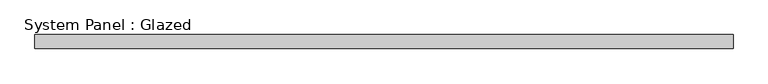
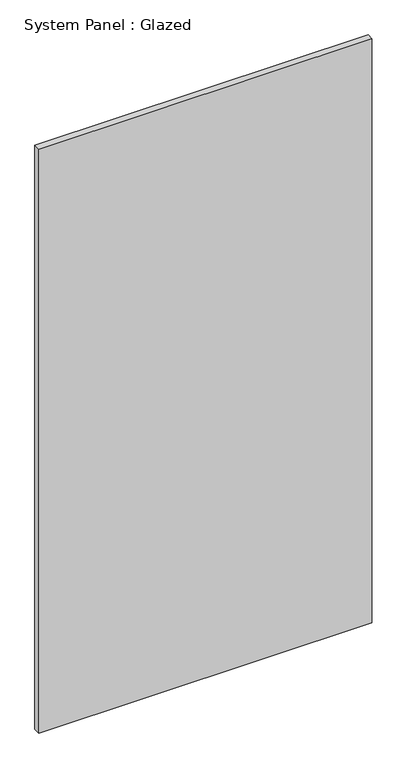
"""IFC4 building model written with IfcOpenShell, lengths in millimetres: plate geometry, System Panel : Glazed."""

from ifc_helpers import new_model, si_unit, origin, origin_with_axes, place, context, project, spatial, polyline, outline, extrude, source, transform, mapped, element, save


def system_panel_glazed_2be43394(model_context):
    return source(origin(), model_context, "Body", "SweptSolid", [
        extrude(outline(polyline([(632.0323546, 19.05), (-632.0323546, 19.05), (-632.0323546, 44.45), (632.0323546, 44.45), (632.0323546, 19.05)])), origin_with_axes(), (0.0, 0.0, 1.0), 2343.15),
    ])


if __name__ == "__main__":
    model = new_model("IFC4")
    model_context = context("Model", 3, world=origin())
    ifc_project = project(units=[si_unit("LENGTHUNIT", "METRE", prefix="MILLI")], contexts=[model_context])
    site = spatial("IfcSite", under=ifc_project)
    building = spatial("IfcBuilding", under=site)
    placement = place(None, origin())
    system_panel_glazed_shape = system_panel_glazed_2be43394(model_context)
    element("IfcPlate", 1, ObjectType="System Panel : Glazed", at=placement, inside=building, context=model_context, shape_type="MappedRepresentation", body=[
        mapped(system_panel_glazed_shape, transform((0.0, 0.0, 0.0), x_axis=(1.0, 0.0, 0.0), y_axis=(0.0, 1.0, 0.0), z_axis=(0.0, 0.0, 1.0))),
    ])
    save(model, "model.ifc")

# Revit data of these elements
# Type "System Panel : Glazed"
#   Construction Type Id = "GSP4R"
#   Analytic Construction = "1/8 in Pilkington single glazing"
#   Visual Light Transmittance = 0.9
#   Solar Heat Gain Coefficient = 0.86
#   Heat Transfer Coefficient (U) = 1.18115 BTU/(h·ft²·°F)
#   Define Thermal Properties by = 1
# Element 1 (IfcPlate, "System Panel : Glazed")
#   Materials on its faces: "Glass"
# Materials
#   "Glass": class "Glass", colour RGB 0 128 192, transparency 0.75, Description = "Soda Lime Glass", Cost = 0
